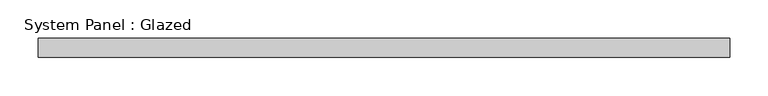
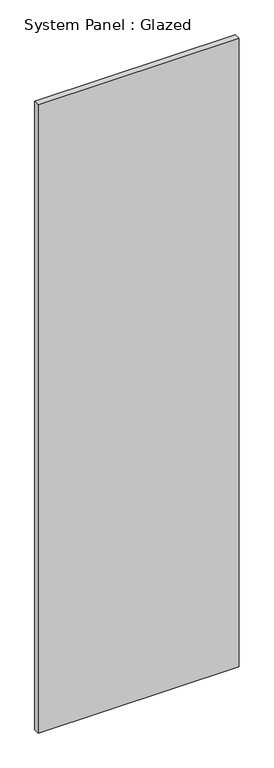
"""IFC4 building model written with IfcOpenShell, lengths in millimetres: plate geometry, System Panel : Glazed."""

from ifc_helpers import new_model, si_unit, origin, origin_with_axes, place, context, project, spatial, polyline, outline, extrude, source, transform, mapped, element, save


def system_panel_glazed_7a5adaf1(model_context):
    return source(origin(), model_context, "Body", "SweptSolid", [
        extrude(outline(polyline([(453.9069819, 24.5), (-453.9069819, 24.5), (-453.9069819, 49.5), (453.9069819, 49.5), (453.9069819, 24.5)])), origin_with_axes(), (0.0, 0.0, 1.0), 3000.0),
    ])


if __name__ == "__main__":
    model = new_model("IFC4")
    model_context = context("Model", 3, world=origin())
    ifc_project = project(units=[si_unit("LENGTHUNIT", "METRE", prefix="MILLI")], contexts=[model_context])
    site = spatial("IfcSite", under=ifc_project)
    building = spatial("IfcBuilding", under=site)
    placement = place(None, origin())
    system_panel_glazed_shape = system_panel_glazed_7a5adaf1(model_context)
    element("IfcPlate", 1, ObjectType="System Panel : Glazed", at=placement, inside=building, context=model_context, shape_type="MappedRepresentation", body=[
        mapped(system_panel_glazed_shape, transform((0.0, 0.0, 0.0), x_axis=(1.0, 0.0, 0.0), y_axis=(0.0, 1.0, 0.0), z_axis=(0.0, 0.0, 1.0))),
    ])
    save(model, "model.ifc")

# Revit data of these elements
# Type "System Panel : Glazed"
#   Keynote = "H11"
#   Construction Type Id = "GSP4R"
#   Analytic Construction = "1/8 in Pilkington single glazing"
#   Visual Light Transmittance = 0.9
#   Solar Heat Gain Coefficient = 0.86
#   Heat Transfer Coefficient (U) = 6.7069 W/(m²·K)
#   Define Thermal Properties by = 1
# Element 1 (IfcPlate, "System Panel : Glazed")
#   Materials on its faces: "Glass"
# Materials
#   "Glass": class "Glass", colour RGB 0 128 192, transparency 0.9, Description = "Soda Lime Glass", Cost = 0
